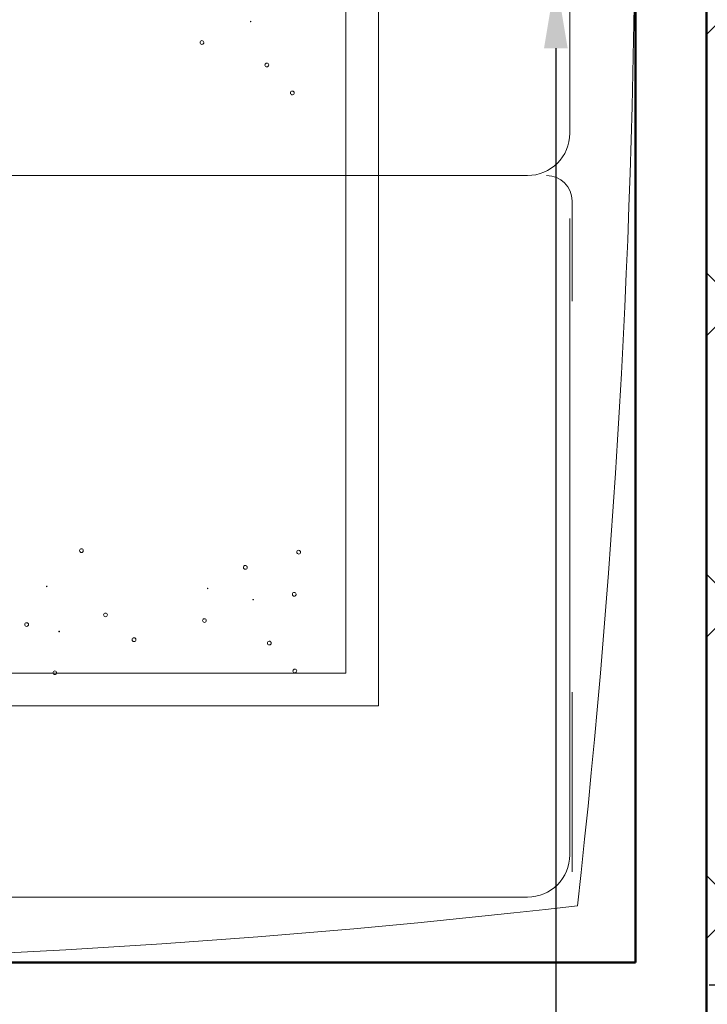
# Model space of a CAD drawing. Units: inches. Extents: x -466983 to 1020, y 324 to 318697.
# Tile 21 of 97: x 775 to 814, y 511 to 566. Entities that reach past the tile are written whole.
import ezdxf

# ---------------------------------------------------------------- set-up
doc = ezdxf.new("R2010")
doc.units = ezdxf.units.IN
doc.header["$MEASUREMENT"] = 0
for name, color, linetype, lineweight in [('A-ANNO-DIMS', 2, 'Continuous', 18), ('A-FLOR-PATT', 252, 'Continuous', 13), ('A-FURN', 8, 'Continuous', 18), ('A-WALL', 7, 'Continuous', 50)]:
    doc.layers.add(name, color=color, linetype=linetype, lineweight=lineweight)
doc.styles.get("Standard").update_dxf_attribs({"font": 'arial.ttf'})
doc.dimstyles.get("Standard").update_dxf_attribs({"dimtxt": 6, "dimasz": 4, "dimexe": 3, "dimexo": 3, "dimgap": 0.09, "dimtad": 0, "dimtih": 1, "dimtoh": 1, "dimdec": 1, "dimzin": 0, "dimdsep": 46, "dimlunit": 3, "dimtxsty": 'Standard', "dimcen": 0.09, "dimadec": 0, "dimazin": 0, "dimtfac": 1, "dimtdec": 1, "dimtofl": 0, "dimtmove": 0, "dimatfit": 3, "dimfxl": 1, "dimtolj": 1, "dimtzin": 0, "dimarcsym": 0})

# ---------------------------------------------------------------- blocks, each defined once
blk = doc.blocks.new('L Shaped Sofa')
at = {"ltscale": 2}
for p, q in [((2475.263, 723.229), (2475.263, 821.686)), ((2458.96, 739.532), (2458.96, 802.773)), ((2460.8, 737.692), (2460.8, 802.773)), ((2471.575, 769.955), (2471.575, 802.773)), ((2469.187, 767.567), (2435.071, 767.567)), ((2471.701, 760.482), (2471.701, 766.134)), ((2471.575, 729.305), (2471.575, 765.138)), ((2458.96, 739.532), (2437.956, 739.532)), ((2471.701, 738.472), (2471.701, 736.259)), ((2460.8, 737.692), (2437.499, 737.692)), ((2471.701, 728.35), (2471.701, 736.259)), ((2469.187, 726.917), (2433.78, 726.917)), ((2475.263, 723.229), (2377.232, 723.229))]:
    blk.add_line(p, q, dxfattribs=at)
for centre, radius, start, end in [((1939.075, 785.436), 536.188, 353.68225, 6.54157), ((2453.608, 776.239), 0.0177, 1.3946, 181.3946), ((2453.608, 776.239), 0.0177, 181.3946, 1.3946), ((2450.866, 775.061), 0.106, 1.3946, 181.3946), ((2450.866, 775.061), 0.106, 181.3946, 1.3946), ((2454.518, 773.793), 0.106, 1.3946, 181.3946), ((2454.518, 773.793), 0.106, 181.3946, 1.3946), ((2455.953, 772.221), 0.106, 1.3946, 181.3946), ((2455.953, 772.221), 0.106, 181.3946, 1.3946), ((2469.187, 769.955), 2.388, 270, 0), ((2470.268, 766.134), 1.433, 0, 90), ((2444.081, 746.436), 0.106, 90, 270), ((2444.081, 746.436), 0.106, 270, 90), ((2456.312, 746.349), 0.106, 1.3946, 181.3946), ((2456.312, 746.349), 0.106, 181.3946, 1.3946), ((2453.309, 745.494), 0.106, 1.3946, 181.3946), ((2453.309, 745.494), 0.106, 181.3946, 1.3946), ((2442.129, 744.423), 0.0177, 90, 270), ((2442.129, 744.423), 0.0177, 270, 90), ((2451.187, 744.312), 0.0177, 1.3946, 181.3946), ((2451.187, 744.312), 0.0177, 181.3946, 1.3946), ((2456.062, 743.978), 0.106, 1.3946, 181.3946), ((2456.062, 743.978), 0.106, 181.3946, 1.3946), ((2453.747, 743.675), 0.0177, 1.3946, 181.3946), ((2453.747, 743.675), 0.0177, 181.3946, 1.3946), ((2445.438, 742.815), 0.106, 90, 270), ((2445.438, 742.815), 0.106, 270, 90), ((2440.998, 742.273), 0.106, 90, 270), ((2440.998, 742.273), 0.106, 270, 90), ((2451.005, 742.498), 0.106, 1.3946, 181.3946), ((2451.005, 742.498), 0.106, 181.3946, 1.3946), ((2442.827, 741.879), 0.0177, 90, 270), ((2442.827, 741.879), 0.0177, 270, 90), ((2447.044, 741.419), 0.106, 90, 270), ((2447.044, 741.419), 0.106, 270, 90), ((2454.657, 741.23), 0.106, 1.3946, 181.3946), ((2454.657, 741.23), 0.106, 181.3946, 1.3946), ((2442.581, 739.558), 0.106, 90, 270), ((2442.581, 739.558), 0.106, 270, 90), ((2456.093, 739.658), 0.106, 1.3946, 181.3946), ((2456.093, 739.658), 0.106, 181.3946, 1.3946), ((2469.187, 729.305), 2.388, 270, 0), ((2416.36, 1205.029), 481.82, 262.88673, 276.63201)]:
    blk.add_arc(centre, radius, start, end, dxfattribs=at)
blk = doc.blocks.new('*D69')
at = {"layer": 'A-ANNO-DIMS', "color": 0, "lineweight": -2, "transparency": 16777216}
for p, q in [((813.968, 636.229), (832.65, 636.229)), ((829.65, 632.229), (829.65, 577.152)), ((829.65, 515.686), (829.65, 570.763)), ((813.968, 511.686), (832.65, 511.686))]:
    blk.add_line(p, q, dxfattribs=at)
at = {"layer": 'A-ANNO-DIMS', "color": 0, "transparency": 16777216}
for points in [[(828.983, 632.229), (830.316, 632.229), (829.65, 636.229)], [(828.983, 515.686), (830.316, 515.686), (829.65, 511.686)]]:
    blk.add_solid(points, dxfattribs=at)
at = {"layer": 'Defpoints', "color": 0, "transparency": 16777216}
for p in [(810.968, 636.229), (829.65, 636.229), (810.968, 511.686)]:
    blk.add_point(p, dxfattribs=at)
at = {"layer": 'A-ANNO-DIMS', "color": 0, "transparency": 16777216, "insert": (829.65, 573.958), "char_height": 6, "attachment_point": 5}
blk.add_mtext('\\A1;L-SOFA 125', dxfattribs=at)
blk = doc.blocks.new('*D70')
at = {"layer": 'A-ANNO-DIMS', "color": 0, "lineweight": -2, "transparency": 16777216}
for p, q in [((689.806, 508.686), (689.806, 490.005)), ((810.968, 508.686), (810.968, 490.005)), ((693.806, 493.005), (744.53, 493.005)), ((806.968, 493.005), (756.244, 493.005))]:
    blk.add_line(p, q, dxfattribs=at)
at = {"layer": 'A-ANNO-DIMS', "color": 0, "transparency": 16777216}
for points in [[(693.806, 493.671), (693.806, 492.338), (689.806, 493.005)], [(806.968, 493.671), (806.968, 492.338), (810.968, 493.005)]]:
    blk.add_solid(points, dxfattribs=at)
at = {"layer": 'Defpoints', "color": 0, "transparency": 16777216}
for p in [(689.806, 511.686), (810.968, 511.686), (810.968, 493.005)]:
    blk.add_point(p, dxfattribs=at)
at = {"layer": 'A-ANNO-DIMS', "color": 0, "transparency": 16777216, "insert": (750.387, 493.005), "char_height": 6, "attachment_point": 5}
blk.add_mtext('\\A1;121', dxfattribs=at)
blk = doc.blocks.new('*D97')
at = {"layer": 'A-ANNO-DIMS', "color": 0, "lineweight": -2, "transparency": 16777216}
for p, q in [((823.929, 568.441), (802.329, 568.441)), ((805.329, 564.441), (805.329, 499.545)), ((805.329, 428.441), (805.329, 493.337)), ((823.929, 424.441), (802.329, 424.441))]:
    blk.add_line(p, q, dxfattribs=at)
at = {"layer": 'A-ANNO-DIMS', "color": 0, "transparency": 16777216}
for points in [[(804.662, 564.441), (805.996, 564.441), (805.329, 568.441)], [(804.662, 428.441), (805.996, 428.441), (805.329, 424.441)]]:
    blk.add_solid(points, dxfattribs=at)
at = {"layer": 'Defpoints', "color": 0, "transparency": 16777216}
for p in [(826.929, 568.441), (805.329, 424.441), (826.929, 424.441)]:
    blk.add_point(p, dxfattribs=at)
at = {"layer": 'A-ANNO-DIMS', "color": 0, "transparency": 16777216, "insert": (805.329, 496.441), "char_height": 6, "attachment_point": 5}
blk.add_mtext('\\A1;BIKE 144', dxfattribs=at)

msp = doc.modelspace()

# ---------------------------------------------------------------- hatches: boundary and pattern name
at = {"layer": 'A-FLOR-PATT', "transparency": 33554572}
h = msp.add_hatch(dxfattribs=at)
h.set_pattern_fill('AR-HBONE', color=256, scale=3)
h.set_pattern_definition([(45, (-1212.414, -290.035), (0, 16.97056), [36, -12]), (135, (-1203.928, -281.55), (1e-15, 16.97056), [36, -12])])
h.paths.add_polyline_path([(987.806, 618.938), (813.806, 618.938), (813.806, 368.938), (987.806, 368.938)])

# ---------------------------------------------------------------- linework, layer by layer
at = {"layer": 'A-WALL'}
for p, q in [((809.806, 655.938), (809.806, 512.938)), ((813.806, 618.938), (813.806, 368.938)), ((809.806, 512.938), (660.806, 512.938))]:
    msp.add_line(p, q, dxfattribs=at)

# ---------------------------------------------------------------- block references
at = {"layer": 'A-FURN'}
msp.add_blockref('L Shaped Sofa', (-1665.457, -210.292), dxfattribs=at)

# ---------------------------------------------------------------- dimensions: what is measured, and where the dimension line sits
at = {"layer": 'A-ANNO-DIMS'}
for base, p1, p2, angle, text, picture, middle in [((829.65, 636.229), (810.968, 511.686), (810.968, 636.229), 90, 'L-SOFA <>', '*D69', (829.65, 573.958)), ((805.329, 424.441), (826.929, 568.441), (826.929, 424.441), 270, 'BIKE <>', '*D97', (805.329, 496.441))]:
    dim = msp.add_linear_dim(base=base, p1=p1, p2=p2, angle=angle, text=text, dimstyle='Standard', override={"dimdec": 0, "dimlfac": 1, "dimrnd": 0, "dimzin": 0, "dimdsep": 46, "dimlunit": 2}, dxfattribs=at)
    dim.commit()
    dim.dimension.update_dxf_attribs({"geometry": picture, "text_midpoint": middle})
dim = msp.add_linear_dim(base=(810.968, 493.005), p1=(689.806, 511.686), p2=(810.968, 511.686), dimstyle='Standard', override={"dimdec": 0, "dimlfac": 1, "dimrnd": 0, "dimzin": 0, "dimdsep": 46, "dimlunit": 2}, dxfattribs=at)
dim.commit()
dim.dimension.update_dxf_attribs({"geometry": '*D70', "text_midpoint": (750.387, 493.005)})

doc.saveas('drawing.dxf')
